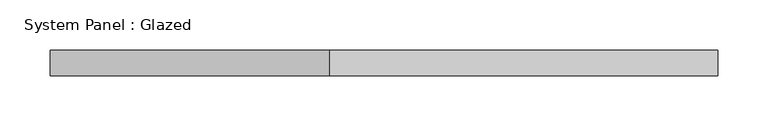
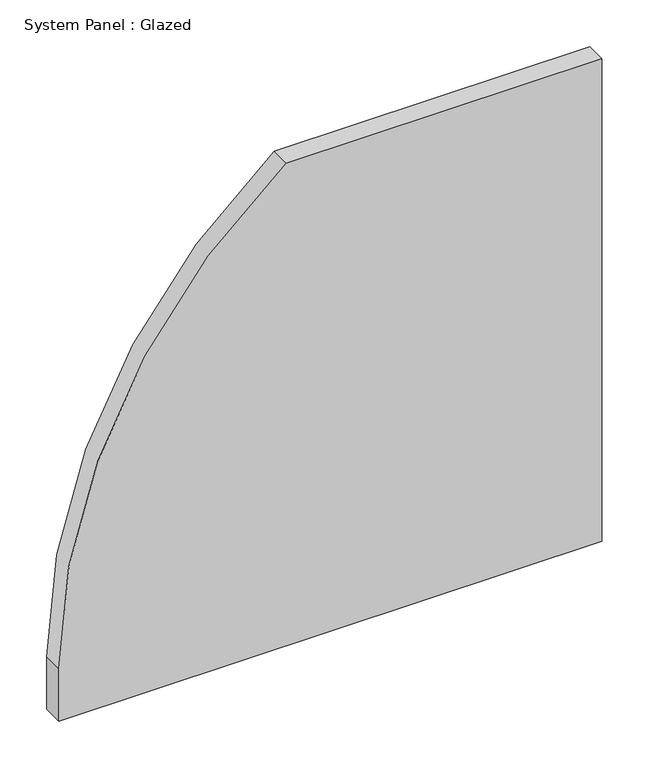
"""IFC4 building model written with IfcOpenShell, lengths in millimetres: plate geometry, System Panel : Glazed."""

from ifc_helpers import new_model, si_unit, point, frame, frame_2d, origin, place, context, project, spatial, polyline, circle_curve, trimmed, segment, composite_curve, outline, extrude, source, transform, mapped, element, save


def system_panel_glazed_4eb050cd(model_context):
    return source(origin(), model_context, "Body", "SweptSolid", [
        extrude(outline(composite_curve([segment(polyline([(0.0, -333.375), (0.0, 333.375), (626.5333333, 333.375), (626.5333333, -53.975)]), True, "CONTINUOUS"), segment(trimmed(circle_curve(frame_2d((67.7333333, 365.125)), 698.5), [point((626.5333333, -53.975))], [point((67.7333333, -333.375))], False, "CARTESIAN"), True, "CONTINUOUS"), segment(polyline([(67.7333333, -333.375), (0.0, -333.375)]), True, "CONTINUOUS")], self_intersect=False)), frame((0.0, 19.05, 0.0), z_axis=(0.0, 1.0, 0.0), x_axis=(0.0, 0.0, 1.0)), (0.0, 0.0, 1.0), 25.4),
    ])


if __name__ == "__main__":
    model = new_model("IFC4")
    model_context = context("Model", 3, world=origin())
    ifc_project = project(units=[si_unit("LENGTHUNIT", "METRE", prefix="MILLI")], contexts=[model_context])
    site = spatial("IfcSite", under=ifc_project)
    building = spatial("IfcBuilding", under=site)
    placement = place(None, origin())
    system_panel_glazed_shape = system_panel_glazed_4eb050cd(model_context)
    element("IfcPlate", 1, ObjectType="System Panel : Glazed", at=placement, inside=building, context=model_context, shape_type="MappedRepresentation", body=[
        mapped(system_panel_glazed_shape, transform((0.0, 0.0, 0.0), x_axis=(1.0, 0.0, 0.0), y_axis=(0.0, 1.0, 0.0), z_axis=(0.0, 0.0, 1.0))),
    ])
    save(model, "model.ifc")

# Revit data of these elements
# Type "System Panel : Glazed"
#   Construction Type Id = "GSP4R"
#   Analytic Construction = "1/8 in Pilkington single glazing"
#   Visual Light Transmittance = 0.9
#   Solar Heat Gain Coefficient = 0.86
#   Heat Transfer Coefficient (U) = 1.18115 BTU/(h·ft²·°F)
#   Define Thermal Properties by = 1
# Element 1 (IfcPlate, "System Panel : Glazed")
#   Materials on its faces: "Glass"
# Materials
#   "Glass": class "Glass", colour RGB 0 128 192, transparency 0.75, Description = "Soda Lime Glass", Cost = 0
